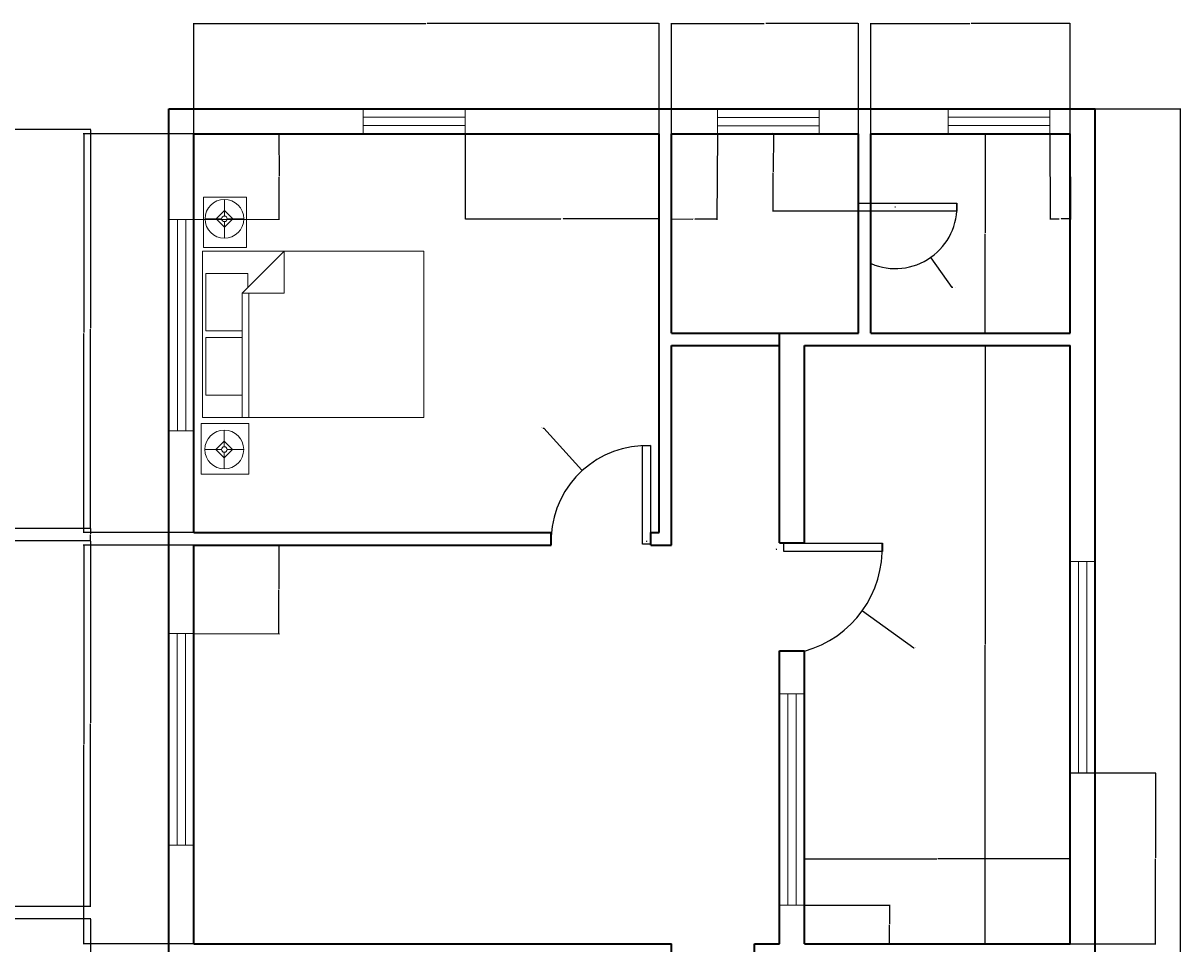
# Model space of a CAD drawing. Units: inches. Extents: x -52 to 1967, y 32 to 824.
# Tile 5 of 10: x 715 to 1133, y 485 to 817. Entities that reach past the tile are written whole.
import ezdxf

# ---------------------------------------------------------------- set-up
doc = ezdxf.new("R2010")
doc.units = ezdxf.units.IN
for name, color, linetype, lineweight in [('A-ANNO-DIMS', 2, 'Continuous', 18), ('A-DOOR', 3, 'Continuous', 25), ('A-FURN', 8, 'Continuous', 18), ('A-GLAZ', 4, 'Continuous', 18), ('A-WALL', 7, 'Continuous', 35)]:
    doc.layers.add(name, color=color, linetype=linetype, lineweight=lineweight)
doc.styles.get("Standard").update_dxf_attribs({"font": 'arial.ttf'})
doc.dimstyles.get("Standard").update_dxf_attribs({"dimtxt": 0.18, "dimasz": 0.18, "dimexe": 0.18, "dimexo": 0.0625, "dimgap": 0.09, "dimtad": 0, "dimtih": 1, "dimtoh": 1, "dimdec": 4, "dimzin": 0, "dimdsep": 46, "dimtxsty": 'Standard', "dimcen": 0.09, "dimadec": 0, "dimazin": 0, "dimtfac": 1, "dimtdec": 4, "dimtofl": 0, "dimtmove": 0, "dimatfit": 3, "dimfxl": 1, "dimtolj": 1, "dimtzin": 0, "dimarcsym": 0})

# ---------------------------------------------------------------- blocks, each defined once
blk = doc.blocks.new('WIN-WIDE-76IN')
for p, q in [((0, 0), (0, 9)), ((0, 9), (76.34, 9)), ((76.34, 9), (76.34, 0)), ((76.34, 6), (0, 6)), ((0, 3), (76.34, 3)), ((76.34, 0), (0, 0))]:
    blk.add_line(p, q)
blk = doc.blocks.new('WIN-NARROW-37IN')
for p, q in [((0, 0), (0, 9)), ((0, 9), (36.78, 9)), ((36.78, 0), (36.78, 9)), ((36.78, 6), (0, 6)), ((0, 3), (36.78, 3)), ((36.78, 0), (0, 0))]:
    blk.add_line(p, q)
blk = doc.blocks.new('DOOR-LEAF-36IN')
blk.add_lwpolyline([(0, 0), (-2.98, 0), (-2.98, 35.63), (0, 35.63)], close=True)
blk = doc.blocks.new('Bed - Queen')
for p, q in [((0, -80.00003), (0, 0)), ((0, 0), (59.99999, 0)), ((59.99999, 0), (59.99999, -80.00003)), ((7.99999, -1.2), (28.79998, -1.2)), ((7.99999, -14.4), (7.99999, -1.2)), ((28.79998, -1.2), (28.79998, -14.4)), ((31.19999, -1.2), (51.99999, -1.2)), ((31.19999, -14.4), (31.19999, -1.2)), ((51.99999, -1.2), (51.99999, -16.4)), ((0, -14.4), (44.8, -14.4)), ((59.99999, -29.6), (44.8, -14.4)), ((44.8, -14.4), (44.8, -29.6)), ((51.99999, -16.4), (46.79936, -16.4)), ((44.8, -16.8), (0, -16.8)), ((44.8, -29.6), (59.99999, -29.6)), ((59.99999, -80.00003), (0, -80.00003))]:
    blk.add_line(p, q)
blk = doc.blocks.new('Lamp - Table')
for p, q in [((0, 7), (0, 1)), ((-1, 0), (-7, 0)), ((0, 3), (-3, 0)), ((-3, 0), (0, -3)), ((3, 0), (0, 3)), ((0, -3), (3, 0)), ((1, 0), (7, 0)), ((0, -1), (0, -7))]:
    blk.add_line(p, q)
for radius in [7, 1]:
    blk.add_circle((0, 0), radius)
blk = doc.blocks.new('BED-QUEEN-WITH-NIGHTSTANDS')
for points in [[(0.4, 61.39), (15.92, 61.39), (15.92, 79.53), (0.4, 79.53)], [(-0.42, -2.26), (16.73, -2.26), (16.73, -20.45), (-0.42, -20.45)]]:
    blk.add_lwpolyline(points, close=True)
for p in [(7.97, 71.69), (7.93, -11.61)]:
    blk.add_blockref('Lamp - Table', p)
at = {"rotation": 90}
blk.add_blockref('Bed - Queen', (0, 0), dxfattribs=at)
blk = doc.blocks.new('*D63')
at = {"layer": 'A-ANNO-DIMS', "color": 0, "lineweight": -2, "transparency": 16777216}
for p, q in [((694.09, 778.97), (739.35, 778.97)), ((739.17, 778.79), (739.17, 707.15)), ((739.17, 635.15), (739.17, 706.79)), ((694.09, 634.97), (739.35, 634.97))]:
    blk.add_line(p, q, dxfattribs=at)
at = {"layer": 'A-ANNO-DIMS', "color": 0, "transparency": 16777216}
for points in [[(739.14, 778.79), (739.2, 778.79), (739.17, 778.97)], [(739.14, 635.15), (739.2, 635.15), (739.17, 634.97)]]:
    blk.add_solid(points, dxfattribs=at)
at = {"layer": 'Defpoints', "color": 0, "transparency": 16777216}
for p in [(694.03, 778.97), (739.17, 778.97), (694.03, 634.97)]:
    blk.add_point(p, dxfattribs=at)
at = {"layer": 'A-ANNO-DIMS', "color": 0, "transparency": 16777216, "insert": (739.17, 706.97), "char_height": 0.18, "attachment_point": 5}
blk.add_mtext('\\A1;144', dxfattribs=at)
blk = doc.blocks.new('*D64')
at = {"layer": 'A-ANNO-DIMS', "color": 0, "lineweight": -2, "transparency": 16777216}
for p, q in [((694.09, 630.47), (739.35, 630.47)), ((739.17, 630.29), (739.17, 564.66)), ((739.17, 498.65), (739.17, 564.29)), ((694.09, 498.47), (739.35, 498.47))]:
    blk.add_line(p, q, dxfattribs=at)
at = {"layer": 'A-ANNO-DIMS', "color": 0, "transparency": 16777216}
for points in [[(739.14, 630.29), (739.2, 630.29), (739.17, 630.47)], [(739.14, 498.65), (739.2, 498.65), (739.17, 498.47)]]:
    blk.add_solid(points, dxfattribs=at)
at = {"layer": 'Defpoints', "color": 0, "transparency": 16777216}
for p in [(694.03, 630.47), (739.17, 630.47), (694.03, 498.47)]:
    blk.add_point(p, dxfattribs=at)
at = {"layer": 'A-ANNO-DIMS', "color": 0, "transparency": 16777216, "insert": (739.17, 564.47), "char_height": 0.18, "attachment_point": 5}
blk.add_mtext('\\A1;132', dxfattribs=at)
blk = doc.blocks.new('*D66')
at = {"layer": 'A-ANNO-DIMS', "color": 0, "lineweight": -2, "transparency": 16777216}
for p, q in [((694.09, 493.97), (739.35, 493.97)), ((739.17, 493.79), (739.17, 434.16)), ((739.17, 374.15), (739.17, 433.79)), ((694.09, 373.97), (739.35, 373.97))]:
    blk.add_line(p, q, dxfattribs=at)
at = {"layer": 'A-ANNO-DIMS', "color": 0, "transparency": 16777216}
for points in [[(739.14, 493.79), (739.2, 493.79), (739.17, 493.97)], [(739.14, 374.15), (739.2, 374.15), (739.17, 373.97)]]:
    blk.add_solid(points, dxfattribs=at)
at = {"layer": 'Defpoints', "color": 0, "transparency": 16777216}
for p in [(694.03, 493.97), (739.17, 493.97), (694.03, 373.97)]:
    blk.add_point(p, dxfattribs=at)
at = {"layer": 'A-ANNO-DIMS', "color": 0, "transparency": 16777216, "insert": (739.17, 433.97), "char_height": 0.18, "attachment_point": 5}
blk.add_mtext('\\A1;120', dxfattribs=at)
blk = doc.blocks.new('*D70')
at = {"layer": 'A-ANNO-DIMS', "color": 0, "lineweight": -2, "transparency": 16777216}
for p, q in [((694.09, 634.97), (739.35, 634.97)), ((739.17, 634.79), (739.17, 632.9)), ((739.17, 630.65), (739.17, 632.54)), ((694.09, 630.47), (739.35, 630.47))]:
    blk.add_line(p, q, dxfattribs=at)
at = {"layer": 'A-ANNO-DIMS', "color": 0, "transparency": 16777216}
for points in [[(739.14, 634.79), (739.2, 634.79), (739.17, 634.97)], [(739.14, 630.65), (739.2, 630.65), (739.17, 630.47)]]:
    blk.add_solid(points, dxfattribs=at)
at = {"layer": 'Defpoints', "color": 0, "transparency": 16777216}
for p in [(694.03, 634.97), (739.17, 634.97), (694.03, 630.47)]:
    blk.add_point(p, dxfattribs=at)
at = {"layer": 'A-ANNO-DIMS', "color": 0, "transparency": 16777216, "insert": (739.17, 632.72), "char_height": 0.18, "attachment_point": 5}
blk.add_mtext('\\A1;4.5', dxfattribs=at)
blk = doc.blocks.new('*D94')
at = {"layer": 'A-ANNO-DIMS', "color": 0, "lineweight": -2, "transparency": 16777216}
for p, q in [((1102.13, 786.35), (1132.97, 786.35)), ((1132.79, 786.17), (1132.79, 480.53)), ((1132.79, 174.53), (1132.79, 480.17)), ((1102.13, 174.35), (1132.97, 174.35))]:
    blk.add_line(p, q, dxfattribs=at)
at = {"layer": 'A-ANNO-DIMS', "color": 0, "transparency": 16777216}
for points in [[(1132.76, 786.17), (1132.82, 786.17), (1132.79, 786.35)], [(1132.76, 174.53), (1132.82, 174.53), (1132.79, 174.35)]]:
    blk.add_solid(points, dxfattribs=at)
at = {"layer": 'Defpoints', "color": 0, "transparency": 16777216}
for p in [(1102.07, 786.35), (1132.79, 786.35), (1102.07, 174.35)]:
    blk.add_point(p, dxfattribs=at)
at = {"layer": 'A-ANNO-DIMS', "color": 0, "transparency": 16777216, "insert": (1132.79, 480.35), "char_height": 0.18, "attachment_point": 5}
blk.add_mtext('\\A1;612', dxfattribs=at)
blk = doc.blocks.new('*D95')
at = {"layer": 'A-ANNO-DIMS', "color": 0, "lineweight": -2, "transparency": 16777216}
for p, q in [((776.57, 777.41), (776.57, 817.28)), ((776.75, 817.1), (860.29, 817.1)), ((944.39, 817.1), (860.85, 817.1)), ((944.57, 777.41), (944.57, 817.28))]:
    blk.add_line(p, q, dxfattribs=at)
at = {"layer": 'A-ANNO-DIMS', "color": 0, "transparency": 16777216}
for points in [[(776.75, 817.13), (776.75, 817.07), (776.57, 817.1)], [(944.39, 817.13), (944.39, 817.07), (944.57, 817.1)]]:
    blk.add_solid(points, dxfattribs=at)
at = {"layer": 'Defpoints', "color": 0, "transparency": 16777216}
for p in [(944.57, 817.1), (776.57, 777.35), (944.57, 777.35)]:
    blk.add_point(p, dxfattribs=at)
at = {"layer": 'A-ANNO-DIMS', "color": 0, "transparency": 16777216, "insert": (860.57, 817.1), "char_height": 0.18, "attachment_point": 5}
blk.add_mtext('\\A1;168', dxfattribs=at)
blk = doc.blocks.new('*D96')
at = {"layer": 'A-ANNO-DIMS', "color": 0, "lineweight": -2, "transparency": 16777216}
for p, q in [((949.07, 777.41), (949.07, 817.28)), ((949.25, 817.1), (982.49, 817.1)), ((1016.39, 817.1), (983.14, 817.1)), ((1016.57, 777.41), (1016.57, 817.28))]:
    blk.add_line(p, q, dxfattribs=at)
at = {"layer": 'A-ANNO-DIMS', "color": 0, "transparency": 16777216}
for points in [[(949.25, 817.13), (949.25, 817.07), (949.07, 817.1)], [(1016.39, 817.13), (1016.39, 817.07), (1016.57, 817.1)]]:
    blk.add_solid(points, dxfattribs=at)
at = {"layer": 'Defpoints', "color": 0, "transparency": 16777216}
for p in [(1016.57, 817.1), (949.07, 777.35), (1016.57, 777.35)]:
    blk.add_point(p, dxfattribs=at)
at = {"layer": 'A-ANNO-DIMS', "color": 0, "transparency": 16777216, "insert": (982.82, 817.1), "char_height": 0.18, "attachment_point": 5}
blk.add_mtext('\\A1;67.5', dxfattribs=at)
blk = doc.blocks.new('*D97')
at = {"layer": 'A-ANNO-DIMS', "color": 0, "lineweight": -2, "transparency": 16777216}
for p, q in [((1021.07, 777.41), (1021.07, 817.28)), ((1021.25, 817.1), (1056.85, 817.1)), ((1092.89, 817.1), (1057.29, 817.1)), ((1093.07, 777.41), (1093.07, 817.28))]:
    blk.add_line(p, q, dxfattribs=at)
at = {"layer": 'A-ANNO-DIMS', "color": 0, "transparency": 16777216}
for points in [[(1021.25, 817.13), (1021.25, 817.07), (1021.07, 817.1)], [(1092.89, 817.13), (1092.89, 817.07), (1093.07, 817.1)]]:
    blk.add_solid(points, dxfattribs=at)
at = {"layer": 'Defpoints', "color": 0, "transparency": 16777216}
for p in [(1093.07, 817.1), (1021.07, 777.35), (1093.07, 777.35)]:
    blk.add_point(p, dxfattribs=at)
at = {"layer": 'A-ANNO-DIMS', "color": 0, "transparency": 16777216, "insert": (1057.07, 817.1), "char_height": 0.18, "attachment_point": 5}
blk.add_mtext('\\A1;72', dxfattribs=at)
blk = doc.blocks.new('*D98')
at = {"layer": 'A-ANNO-DIMS', "color": 0, "lineweight": -2, "transparency": 16777216}
for p, q in [((776.51, 777.35), (736.6, 777.35)), ((736.78, 777.17), (736.78, 705.53)), ((736.78, 633.53), (736.78, 705.17)), ((776.51, 633.35), (736.6, 633.35))]:
    blk.add_line(p, q, dxfattribs=at)
at = {"layer": 'A-ANNO-DIMS', "color": 0, "transparency": 16777216}
for points in [[(736.75, 777.17), (736.81, 777.17), (736.78, 777.35)], [(736.75, 633.53), (736.81, 633.53), (736.78, 633.35)]]:
    blk.add_solid(points, dxfattribs=at)
at = {"layer": 'Defpoints', "color": 0, "transparency": 16777216}
for p in [(736.78, 777.35), (776.57, 777.35), (776.57, 633.35)]:
    blk.add_point(p, dxfattribs=at)
at = {"layer": 'A-ANNO-DIMS', "color": 0, "transparency": 16777216, "insert": (736.78, 705.35), "char_height": 0.18, "attachment_point": 5}
blk.add_mtext('\\A1;144', dxfattribs=at)
blk = doc.blocks.new('*D99')
at = {"layer": 'A-ANNO-DIMS', "color": 0, "lineweight": -2, "transparency": 16777216}
for p, q in [((1093.01, 777.35), (1062.16, 777.35)), ((1062.34, 777.17), (1062.34, 741.53)), ((1062.34, 705.53), (1062.34, 741.17)), ((1093.01, 705.35), (1062.16, 705.35))]:
    blk.add_line(p, q, dxfattribs=at)
at = {"layer": 'A-ANNO-DIMS', "color": 0, "transparency": 16777216}
for points in [[(1062.31, 777.17), (1062.37, 777.17), (1062.34, 777.35)], [(1062.31, 705.53), (1062.37, 705.53), (1062.34, 705.35)]]:
    blk.add_solid(points, dxfattribs=at)
at = {"layer": 'Defpoints', "color": 0, "transparency": 16777216}
for p in [(1062.34, 777.35), (1093.07, 777.35), (1093.07, 705.35)]:
    blk.add_point(p, dxfattribs=at)
at = {"layer": 'A-ANNO-DIMS', "color": 0, "transparency": 16777216, "insert": (1062.34, 741.35), "char_height": 0.18, "attachment_point": 5}
blk.add_mtext('\\A1;72', dxfattribs=at)
blk = doc.blocks.new('*D100')
at = {"layer": 'A-ANNO-DIMS', "color": 0, "lineweight": -2, "transparency": 16777216}
for p, q in [((1093.01, 700.85), (1062.16, 700.85)), ((1062.34, 700.67), (1062.34, 593.03)), ((1062.34, 485.03), (1062.34, 592.67)), ((1093.01, 484.85), (1062.16, 484.85))]:
    blk.add_line(p, q, dxfattribs=at)
at = {"layer": 'A-ANNO-DIMS', "color": 0, "transparency": 16777216}
for points in [[(1062.31, 700.67), (1062.37, 700.67), (1062.34, 700.85)], [(1062.31, 485.03), (1062.37, 485.03), (1062.34, 484.85)]]:
    blk.add_solid(points, dxfattribs=at)
at = {"layer": 'Defpoints', "color": 0, "transparency": 16777216}
for p in [(1062.34, 700.85), (1093.07, 700.85), (1093.07, 484.85)]:
    blk.add_point(p, dxfattribs=at)
at = {"layer": 'A-ANNO-DIMS', "color": 0, "transparency": 16777216, "insert": (1062.34, 592.85), "char_height": 0.18, "attachment_point": 5}
blk.add_mtext('\\A1;216', dxfattribs=at)
blk = doc.blocks.new('*D101')
at = {"layer": 'A-ANNO-DIMS', "color": 0, "lineweight": -2, "transparency": 16777216}
for p, q in [((776.51, 628.85), (736.6, 628.85)), ((736.78, 628.67), (736.78, 557.03)), ((736.78, 485.03), (736.78, 556.67)), ((776.51, 484.85), (736.6, 484.85))]:
    blk.add_line(p, q, dxfattribs=at)
at = {"layer": 'A-ANNO-DIMS', "color": 0, "transparency": 16777216}
for points in [[(736.75, 628.67), (736.81, 628.67), (736.78, 628.85)], [(736.75, 485.03), (736.81, 485.03), (736.78, 484.85)]]:
    blk.add_solid(points, dxfattribs=at)
at = {"layer": 'Defpoints', "color": 0, "transparency": 16777216}
for p in [(736.78, 628.85), (776.57, 628.85), (776.57, 484.85)]:
    blk.add_point(p, dxfattribs=at)
at = {"layer": 'A-ANNO-DIMS', "color": 0, "transparency": 16777216, "insert": (736.78, 556.85), "char_height": 0.18, "attachment_point": 5}
blk.add_mtext('\\A1;144', dxfattribs=at)
blk = doc.blocks.new('*D105')
at = {"layer": 'A-ANNO-DIMS', "color": 0, "lineweight": -2, "transparency": 16777216}
for p, q in [((997.07, 484.91), (997.07, 515.75)), ((997.25, 515.57), (1044.85, 515.57)), ((1092.89, 515.57), (1045.29, 515.57)), ((1093.07, 484.91), (1093.07, 515.75))]:
    blk.add_line(p, q, dxfattribs=at)
at = {"layer": 'A-ANNO-DIMS', "color": 0, "transparency": 16777216}
for points in [[(997.25, 515.6), (997.25, 515.54), (997.07, 515.57)], [(1092.89, 515.6), (1092.89, 515.54), (1093.07, 515.57)]]:
    blk.add_solid(points, dxfattribs=at)
at = {"layer": 'Defpoints', "color": 0, "transparency": 16777216}
for p in [(1093.07, 515.57), (997.07, 484.85), (1093.07, 484.85)]:
    blk.add_point(p, dxfattribs=at)
at = {"layer": 'A-ANNO-DIMS', "color": 0, "transparency": 16777216, "insert": (1045.07, 515.57), "char_height": 0.18, "attachment_point": 5}
blk.add_mtext('\\A1;96', dxfattribs=at)
blk = doc.blocks.new('*D107')
at = {"layer": 'A-ANNO-DIMS', "color": 0, "lineweight": -2, "transparency": 16777216}
for p, q in [((874.48, 777.32), (874.47, 746.47)), ((944.57, 777.29), (944.56, 746.44)), ((874.65, 746.65), (909.12, 746.64)), ((944.38, 746.62), (909.91, 746.64))]:
    blk.add_line(p, q, dxfattribs=at)
at = {"layer": 'A-ANNO-DIMS', "color": 0, "transparency": 16777216}
for points in [[(874.65, 746.68), (874.65, 746.62), (874.47, 746.65)], [(944.38, 746.65), (944.38, 746.59), (944.56, 746.62)]]:
    blk.add_solid(points, dxfattribs=at)
at = {"layer": 'Defpoints', "color": 0, "transparency": 16777216}
for p in [(874.48, 777.38), (944.57, 777.35), (874.47, 746.65)]:
    blk.add_point(p, dxfattribs=at)
at = {"layer": 'A-ANNO-DIMS', "color": 0, "transparency": 16777216, "insert": (909.51, 746.64), "char_height": 0.18, "attachment_point": 5}
blk.add_mtext('\\A1;70.09', dxfattribs=at)
blk = doc.blocks.new('*D108')
at = {"layer": 'A-ANNO-DIMS', "color": 0, "lineweight": -2, "transparency": 16777216}
for p, q in [((949.07, 777.29), (948.83, 746.44)), ((965.62, 777.16), (965.38, 746.32)), ((949.01, 746.62), (956.72, 746.56)), ((965.2, 746.5), (957.49, 746.56))]:
    blk.add_line(p, q, dxfattribs=at)
at = {"layer": 'A-ANNO-DIMS', "color": 0, "transparency": 16777216}
for points in [[(949.01, 746.65), (949.01, 746.59), (948.83, 746.62)], [(965.2, 746.53), (965.2, 746.47), (965.38, 746.5)]]:
    blk.add_solid(points, dxfattribs=at)
at = {"layer": 'Defpoints', "color": 0, "transparency": 16777216}
for p in [(949.07, 777.35), (965.62, 777.22), (948.83, 746.62)]:
    blk.add_point(p, dxfattribs=at)
at = {"layer": 'A-ANNO-DIMS', "color": 0, "transparency": 16777216, "insert": (957.1, 746.56), "char_height": 0.18, "attachment_point": 5}
blk.add_mtext('\\A1;16.55', dxfattribs=at)
blk = doc.blocks.new('*D109')
at = {"layer": 'A-ANNO-DIMS', "color": 0, "lineweight": -2, "transparency": 16777216}
for p, q in [((1085.7, 777.27), (1085.77, 746.43)), ((1093.07, 777.29), (1093.14, 746.44)), ((1085.95, 746.61), (1089.08, 746.61)), ((1092.96, 746.62), (1089.83, 746.62))]:
    blk.add_line(p, q, dxfattribs=at)
at = {"layer": 'A-ANNO-DIMS', "color": 0, "transparency": 16777216}
for points in [[(1085.95, 746.64), (1085.95, 746.58), (1085.77, 746.61)], [(1092.96, 746.65), (1092.96, 746.59), (1093.14, 746.62)]]:
    blk.add_solid(points, dxfattribs=at)
at = {"layer": 'Defpoints', "color": 0, "transparency": 16777216}
for p in [(1085.7, 777.33), (1093.07, 777.35), (1085.77, 746.61)]:
    blk.add_point(p, dxfattribs=at)
at = {"layer": 'A-ANNO-DIMS', "color": 0, "transparency": 16777216, "insert": (1089.45, 746.61), "char_height": 0.18, "attachment_point": 5}
blk.add_mtext('\\A1;7.371', dxfattribs=at)
blk = doc.blocks.new('*D112')
at = {"layer": 'A-ANNO-DIMS', "color": 0, "lineweight": -2, "transparency": 16777216}
for p, q in [((776.63, 777.35), (807.47, 777.37)), ((807.29, 777.19), (807.3, 762.09)), ((807.31, 746.64), (807.3, 761.73)), ((776.65, 746.44), (807.49, 746.46))]:
    blk.add_line(p, q, dxfattribs=at)
at = {"layer": 'A-ANNO-DIMS', "color": 0, "transparency": 16777216}
for points in [[(807.32, 777.19), (807.26, 777.19), (807.29, 777.37)], [(807.34, 746.64), (807.28, 746.64), (807.31, 746.46)]]:
    blk.add_solid(points, dxfattribs=at)
at = {"layer": 'Defpoints', "color": 0, "transparency": 16777216}
for p in [(776.57, 777.35), (776.59, 746.44), (807.31, 746.46)]:
    blk.add_point(p, dxfattribs=at)
at = {"layer": 'A-ANNO-DIMS', "color": 0, "transparency": 16777216, "insert": (807.3, 761.91), "char_height": 0.18, "attachment_point": 5}
blk.add_mtext('\\A1;30.91', dxfattribs=at)
blk = doc.blocks.new('*D113')
at = {"layer": 'A-ANNO-DIMS', "color": 0, "lineweight": -2, "transparency": 16777216}
for p, q in [((776.63, 628.85), (807.47, 628.82)), ((807.29, 628.64), (807.28, 613)), ((807.26, 596.99), (807.28, 612.63)), ((776.6, 596.84), (807.44, 596.81))]:
    blk.add_line(p, q, dxfattribs=at)
at = {"layer": 'A-ANNO-DIMS', "color": 0, "transparency": 16777216}
for points in [[(807.26, 628.64), (807.32, 628.64), (807.29, 628.82)], [(807.23, 596.99), (807.29, 596.99), (807.26, 596.81)]]:
    blk.add_solid(points, dxfattribs=at)
at = {"layer": 'Defpoints', "color": 0, "transparency": 16777216}
for p in [(776.57, 628.85), (776.54, 596.84), (807.26, 596.81)]:
    blk.add_point(p, dxfattribs=at)
at = {"layer": 'A-ANNO-DIMS', "color": 0, "transparency": 16777216, "insert": (807.28, 612.81), "char_height": 0.18, "attachment_point": 5}
blk.add_mtext('\\A1;32.005', dxfattribs=at)
blk = doc.blocks.new('*D115')
at = {"layer": 'A-ANNO-DIMS', "color": 0, "lineweight": -2, "transparency": 16777216}
for p, q in [((997.12, 498.79), (1027.96, 498.82)), ((1027.78, 498.64), (1027.79, 492.03)), ((1027.79, 485.06), (1027.79, 491.66)), ((997.13, 484.85), (1027.97, 484.88))]:
    blk.add_line(p, q, dxfattribs=at)
at = {"layer": 'A-ANNO-DIMS', "color": 0, "transparency": 16777216}
for points in [[(1027.81, 498.64), (1027.75, 498.64), (1027.78, 498.82)], [(1027.82, 485.06), (1027.76, 485.06), (1027.79, 484.88)]]:
    blk.add_solid(points, dxfattribs=at)
at = {"layer": 'Defpoints', "color": 0, "transparency": 16777216}
for p in [(997.06, 498.79), (997.07, 484.85), (1027.79, 484.88)]:
    blk.add_point(p, dxfattribs=at)
at = {"layer": 'A-ANNO-DIMS', "color": 0, "transparency": 16777216, "insert": (1027.79, 491.85), "char_height": 0.18, "attachment_point": 5}
blk.add_mtext('\\A1;13.937', dxfattribs=at)
blk = doc.blocks.new('*D117')
at = {"layer": 'A-ANNO-DIMS', "color": 0, "lineweight": -2, "transparency": 16777216}
for p, q in [((1093.13, 546.61), (1123.97, 546.62)), ((1123.79, 546.44), (1123.79, 515.91)), ((1123.79, 485.03), (1123.79, 515.55)), ((1093.13, 484.85), (1123.97, 484.85))]:
    blk.add_line(p, q, dxfattribs=at)
at = {"layer": 'A-ANNO-DIMS', "color": 0, "transparency": 16777216}
for points in [[(1123.82, 546.44), (1123.76, 546.44), (1123.79, 546.62)], [(1123.82, 485.03), (1123.76, 485.03), (1123.79, 484.85)]]:
    blk.add_solid(points, dxfattribs=at)
at = {"layer": 'Defpoints', "color": 0, "transparency": 16777216}
for p in [(1093.06, 546.61), (1093.07, 484.85), (1123.79, 484.85)]:
    blk.add_point(p, dxfattribs=at)
at = {"layer": 'A-ANNO-DIMS', "color": 0, "transparency": 16777216, "insert": (1123.79, 515.73), "char_height": 0.18, "attachment_point": 5}
blk.add_mtext('\\A1;61.76', dxfattribs=at)
blk = doc.blocks.new('*D119')
at = {"layer": 'A-ANNO-DIMS', "color": 0, "lineweight": -2, "transparency": 16777216}
for p, q in [((1016.51, 777.35), (985.66, 777.46)), ((985.84, 777.28), (985.8, 763.64)), ((985.75, 749.63), (985.79, 763.27)), ((1016.41, 749.34), (985.57, 749.45))]:
    blk.add_line(p, q, dxfattribs=at)
at = {"layer": 'A-ANNO-DIMS', "color": 0, "transparency": 16777216}
for points in [[(985.81, 777.28), (985.87, 777.28), (985.84, 777.46)], [(985.72, 749.63), (985.78, 749.63), (985.75, 749.45)]]:
    blk.add_solid(points, dxfattribs=at)
at = {"layer": 'Defpoints', "color": 0, "transparency": 16777216}
for p in [(985.84, 777.46), (1016.57, 777.35), (1016.47, 749.34)]:
    blk.add_point(p, dxfattribs=at)
at = {"layer": 'A-ANNO-DIMS', "color": 0, "transparency": 16777216, "insert": (985.79, 763.45), "char_height": 0.18, "attachment_point": 5}
blk.add_mtext('\\A1;28.004', dxfattribs=at)
blk = doc.blocks.new('*D142')
at = {"layer": 'A-ANNO-DIMS', "color": 0, "lineweight": -2, "transparency": 16777216}
for p, q in [((986.85, 627.39), (987.03, 627.39)), ((986.94, 627.3), (986.94, 627.48)), ((1036.52, 591.64), (1018.07, 604.94)), ((1036.7, 591.64), (1036.52, 591.64))]:
    blk.add_line(p, q, dxfattribs=at)
at = {"layer": 'A-ANNO-DIMS', "color": 0, "transparency": 16777216}
blk.add_solid([(1018.09, 604.96), (1018.06, 604.91), (1017.93, 605.04)], dxfattribs=at)
at = {"layer": 'Defpoints', "color": 0, "transparency": 16777216}
for p in [(986.94, 627.39), (1017.93, 605.04)]:
    blk.add_point(p, dxfattribs=at)
at = {"layer": 'A-ANNO-DIMS', "color": 0, "transparency": 16777216, "insert": (1037.11, 591.64), "char_height": 0.18, "attachment_point": 5}
blk.add_mtext('\\A1;R38.2', dxfattribs=at)
blk = doc.blocks.new('*D143')
at = {"layer": 'A-ANNO-DIMS', "color": 0, "lineweight": -2, "transparency": 16777216}
for p, q in [((902.71, 671.08), (902.89, 671.08)), ((902.89, 671.08), (916.72, 655.89)), ((940.01, 630.21), (940.19, 630.21)), ((940.1, 630.12), (940.1, 630.3))]:
    blk.add_line(p, q, dxfattribs=at)
at = {"layer": 'A-ANNO-DIMS', "color": 0, "transparency": 16777216}
blk.add_solid([(916.75, 655.91), (916.7, 655.87), (916.84, 655.75)], dxfattribs=at)
at = {"layer": 'Defpoints', "color": 0, "transparency": 16777216}
for p in [(916.84, 655.75), (940.1, 630.21)]:
    blk.add_point(p, dxfattribs=at)
at = {"layer": 'A-ANNO-DIMS', "color": 0, "transparency": 16777216, "insert": (902.23, 671.08), "char_height": 0.18, "attachment_point": 5}
blk.add_mtext('\\A1;R34.54', dxfattribs=at)
blk = doc.blocks.new('*D147')
at = {"layer": 'A-ANNO-DIMS', "color": 0, "lineweight": -2, "transparency": 16777216}
for p, q in [((1029.78, 750.92), (1029.96, 750.92)), ((1029.87, 750.83), (1029.87, 751.01)), ((1050.42, 721.81), (1042.82, 732.58)), ((1050.6, 721.81), (1050.42, 721.81))]:
    blk.add_line(p, q, dxfattribs=at)
at = {"layer": 'A-ANNO-DIMS', "color": 0, "transparency": 16777216}
blk.add_solid([(1042.84, 732.6), (1042.79, 732.56), (1042.71, 732.73)], dxfattribs=at)
at = {"layer": 'Defpoints', "color": 0, "transparency": 16777216}
for p in [(1029.87, 750.92), (1042.71, 732.73)]:
    blk.add_point(p, dxfattribs=at)
at = {"layer": 'A-ANNO-DIMS', "color": 0, "transparency": 16777216, "insert": (1051.15, 721.81), "char_height": 0.18, "attachment_point": 5}
blk.add_mtext('\\A1;R22.266', dxfattribs=at)

msp = doc.modelspace()

# ---------------------------------------------------------------- linework, layer by layer
at = {"layer": 'A-DOOR'}
for centre, radius, start, end in [((1029.8747, 750.9197), 22.2655, 246.819309, 3.604465), ((940.0996, 630.2128), 34.5415, 87.650237, 176.986288), ((986.9404, 627.3896), 38.2029, 285.312902, 3.09422)]:
    msp.add_arc(centre, radius, start, end, dxfattribs=at)
at = {"layer": 'A-WALL'}
for p, q in [((767.5687, 786.3484), (1102.0687, 786.3484)), ((767.5687, 174.3484), (767.5687, 786.3484)), ((1102.0687, 174.3484), (1102.0687, 786.3484)), ((776.5687, 777.3484), (944.5687, 777.3484)), ((776.5687, 633.3484), (776.5687, 777.3484)), ((944.5687, 633.3484), (944.5687, 777.3484)), ((949.0687, 705.3484), (949.0687, 777.3484)), ((949.0687, 777.3484), (1016.5687, 777.3484)), ((1016.5687, 705.3484), (1016.5687, 777.3484)), ((1021.0687, 705.3484), (1021.0687, 777.3484)), ((1021.0687, 777.3484), (1093.0687, 777.3484)), ((1093.0687, 705.3484), (1093.0687, 777.3484)), ((949.0687, 705.3484), (1016.5687, 705.3484)), ((988.0687, 629.5782), (988.0687, 705.3484)), ((1021.0687, 705.3484), (1093.0687, 705.3484)), ((949.0687, 700.8484), (988.0687, 700.8484)), ((949.0687, 628.8484), (949.0687, 700.8484)), ((997.0687, 700.8484), (1093.0687, 700.8484)), ((997.0687, 629.5782), (997.0687, 700.8484)), ((1093.0687, 484.8484), (1093.0687, 700.8484)), ((776.5687, 633.3484), (905.5687, 633.3484)), ((905.5687, 628.8484), (905.5687, 633.3484)), ((941.5687, 628.8484), (941.5687, 633.3484)), ((941.5687, 633.3484), (944.5687, 633.3484)), ((776.5687, 628.8484), (905.5687, 628.8484)), ((776.5687, 484.8484), (776.5687, 628.8484)), ((941.5687, 628.8484), (949.0687, 628.8484)), ((988.0687, 629.5782), (997.0687, 629.5782)), ((988.0687, 484.8484), (988.0687, 590.5782)), ((988.0687, 590.5782), (997.0687, 590.5782)), ((997.0687, 484.8484), (997.0687, 590.5782)), ((776.5687, 484.8484), (949.0687, 484.8484)), ((949.0687, 477.3484), (949.0687, 484.8484)), ((979.0687, 484.8484), (988.0687, 484.8484)), ((979.0687, 480.3484), (979.0687, 484.8484)), ((997.0687, 484.8484), (1093.0687, 484.8484))]:
    msp.add_line(p, q, dxfattribs=at)

# ---------------------------------------------------------------- block references
at = {"layer": 'A-DOOR'}
for p, rotation in [((1016.4702, 749.3441), 269.9999999999998), ((989.5832, 626.5098), 269.9999999999999)]:
    msp.add_blockref('DOOR-LEAF-36IN', p, dxfattribs=dict(at, rotation=rotation))
msp.add_blockref('DOOR-LEAF-36IN', (941.5227, 629.1009), dxfattribs=at)
at = {"layer": 'A-FURN'}
msp.add_blockref('BED-QUEEN-WITH-NIGHTSTANDS', (779.6128, 674.9358), dxfattribs=at)
at = {"layer": 'A-GLAZ'}
for p in [(837.7008, 777.3784), (965.6176, 777.2195), (1048.9162, 777.3313)]:
    msp.add_blockref('WIN-NARROW-37IN', p, dxfattribs=at)
for p, rotation in [((767.5884, 746.4361), 270), ((1093.0641, 622.9533), 270), ((767.5352, 596.8439), 270), ((988.0554, 575.1259), 269.9999999999998)]:
    msp.add_blockref('WIN-WIDE-76IN', p, dxfattribs=dict(at, rotation=rotation))

# ---------------------------------------------------------------- dimensions: what is measured, and where the dimension line sits
at = {"layer": 'A-ANNO-DIMS'}
for base, p1, p2, override, picture, middle in [((944.5687, 817.1034), (776.5687, 777.3484), (944.5687, 777.3484), {"dimdec": 0, "dimlfac": 1, "dimrnd": 0, "dimzin": 0, "dimdsep": 46, "dimlunit": 2}, '*D95', (860.5687, 817.1034)), ((1016.5687, 817.1034), (949.0687, 777.3484), (1016.5687, 777.3484), {"dimdec": 1, "dimlfac": 1, "dimrnd": 0, "dimzin": 0, "dimdsep": 46, "dimlunit": 2}, '*D96', (982.8187, 817.1034)), ((1093.0687, 817.1034), (1021.0687, 777.3484), (1093.0687, 777.3484), {"dimdec": 0, "dimlfac": 1, "dimrnd": 0, "dimzin": 0, "dimdsep": 46, "dimlunit": 2}, '*D97', (1057.0687, 817.1034)), ((1093.0687, 515.5734), (997.0687, 484.8484), (1093.0687, 484.8484), {"dimdec": 0, "dimlfac": 1, "dimrnd": 0, "dimzin": 0, "dimdsep": 46, "dimlunit": 2}, '*D105', (1045.0687, 515.5734))]:
    dim = msp.add_linear_dim(base=base, p1=p1, p2=p2, dimstyle='Standard', override=override, dxfattribs=at)
    dim.commit()
    dim.dimension.update_dxf_attribs({"geometry": picture, "text_midpoint": middle})
for base, p1, p2, angle, override, picture, middle in [((1132.7937, 786.3484), (1102.0687, 174.3484), (1102.0687, 786.3484), 90, {"dimdec": 0, "dimlfac": 1, "dimrnd": 0, "dimzin": 0, "dimdsep": 46, "dimlunit": 2}, '*D94', (1132.7937, 480.3484)), ((739.1728, 778.9731), (694.0273, 634.9731), (694.0273, 778.9731), 90, {"dimdec": 0, "dimlfac": 1, "dimrnd": 0, "dimzin": 0, "dimdsep": 46, "dimlunit": 2}, '*D63', (739.1728, 706.9731)), ((736.7792, 777.3484), (776.5687, 633.3484), (776.5687, 777.3484), 90, {"dimdec": 0, "dimlfac": 1, "dimrnd": 0, "dimzin": 0, "dimdsep": 46, "dimlunit": 2}, '*D98', (736.7792, 705.3484)), ((807.3134, 746.4557), (776.5687, 777.3484), (776.5884, 746.4361), 270.036507, {"dimdec": 2, "dimlfac": 1, "dimrnd": 0, "dimzin": 0, "dimdsep": 46, "dimlunit": 2}, '*D112', (807.3036, 761.9119)), ((874.4693, 746.6534), (944.5687, 777.3484), (874.4825, 777.3784), 179.975476, {"dimdec": 2, "dimlfac": 1, "dimrnd": 0, "dimzin": 0, "dimdsep": 46, "dimlunit": 2}, '*D107', (909.5125, 746.6384)), ((948.8293, 746.6244), (965.6176, 777.2195), (949.0687, 777.3484), 179.553561, {"dimdec": 2, "dimlfac": 1, "dimrnd": 0, "dimzin": 0, "dimdsep": 46, "dimlunit": 2}, '*D108', (957.1037, 746.5599)), ((985.8439, 777.4565), (1016.4702, 749.3441), (1016.5687, 777.3484), 89.79851, {"dimdec": 3, "dimlfac": 1, "dimrnd": 0, "dimzin": 0, "dimdsep": 46, "dimlunit": 2}, '*D119', (985.7947, 763.4543)), ((1062.3437, 777.3484), (1093.0687, 705.3484), (1093.0687, 777.3484), 90, {"dimdec": 0, "dimlfac": 1, "dimrnd": 0, "dimzin": 0, "dimdsep": 46, "dimlunit": 2}, '*D99', (1062.3437, 741.3484)), ((1085.7692, 746.6064), (1093.0687, 777.3484), (1085.6979, 777.3313), 180.133009, {"dimdec": 3, "dimlfac": 1, "dimrnd": 0, "dimzin": 0, "dimdsep": 46, "dimlunit": 2}, '*D109', (1089.4546, 746.615)), ((1062.3437, 700.8484), (1093.0687, 484.8484), (1093.0687, 700.8484), 90, {"dimdec": 0, "dimlfac": 1, "dimrnd": 0, "dimzin": 0, "dimdsep": 46, "dimlunit": 2}, '*D100', (1062.3437, 592.8484)), ((739.1728, 634.9731), (694.0273, 630.4731), (694.0273, 634.9731), 90, {"dimdec": 1, "dimlfac": 1, "dimrnd": 0, "dimzin": 0, "dimdsep": 46, "dimlunit": 2}, '*D70', (739.1728, 632.7231)), ((739.1728, 630.4731), (694.0273, 498.4731), (694.0273, 630.4731), 90, {"dimdec": 0, "dimlfac": 1, "dimrnd": 0, "dimzin": 0, "dimdsep": 46, "dimlunit": 2}, '*D64', (739.1728, 564.4731)), ((736.7792, 628.8484), (776.5687, 484.8484), (776.5687, 628.8484), 90, {"dimdec": 0, "dimlfac": 1, "dimrnd": 0, "dimzin": 0, "dimdsep": 46, "dimlunit": 2}, '*D101', (736.7792, 556.8484)), ((807.2602, 596.8118), (776.5687, 628.8484), (776.5352, 596.8439), 269.940052, {"dimdec": 3, "dimlfac": 1, "dimrnd": 0, "dimzin": 0, "dimdsep": 46, "dimlunit": 2}, '*D113', (807.277, 612.814)), ((1123.7937, 484.8507), (1093.0641, 546.6131), (1093.0687, 484.8484), 270.004248, {"dimdec": 2, "dimlfac": 1, "dimrnd": 0, "dimzin": 0, "dimdsep": 46, "dimlunit": 2}, '*D117', (1123.7914, 515.733)), ((1027.7937, 484.8779), (997.0554, 498.7858), (997.0687, 484.8484), 270.05492, {"dimdec": 3, "dimlfac": 1, "dimrnd": 0, "dimzin": 0, "dimdsep": 46, "dimlunit": 2}, '*D115', (1027.787, 491.8466)), ((739.1728, 493.9731), (694.0273, 373.9731), (694.0273, 493.9731), 90, {"dimdec": 0, "dimlfac": 1, "dimrnd": 0, "dimzin": 0, "dimdsep": 46, "dimlunit": 2}, '*D66', (739.1728, 433.9731))]:
    dim = msp.add_linear_dim(base=base, p1=p1, p2=p2, angle=angle, dimstyle='Standard', override=override, dxfattribs=at)
    dim.commit()
    dim.dimension.update_dxf_attribs({"geometry": picture, "text_midpoint": middle})
for center, mpoint, override, picture, middle in [((1029.8747, 750.9197), (1042.7129, 732.7281), {"dimdec": 3, "dimlfac": 1, "dimrnd": 0, "dimzin": 0, "dimdsep": 46, "dimlunit": 2}, '*D147', (1051.1456, 721.8132)), ((940.0996, 630.2128), (916.8447, 655.7534), {"dimdec": 2, "dimlfac": 1, "dimrnd": 0, "dimzin": 0, "dimdsep": 46, "dimlunit": 2}, '*D143', (902.2322, 671.0777)), ((986.9404, 627.3896), (1017.9266, 605.0443), {"dimdec": 1, "dimlfac": 1, "dimrnd": 0, "dimzin": 0, "dimdsep": 46, "dimlunit": 2}, '*D142', (1037.1073, 591.6371))]:
    dim = msp.add_radius_dim(center=center, mpoint=mpoint, dimstyle='Standard', override=override, dxfattribs=at)
    dim.commit()
    dim.dimension.update_dxf_attribs({"geometry": picture, "text_midpoint": middle, "dimtype": 164})

doc.saveas('drawing.dxf')
